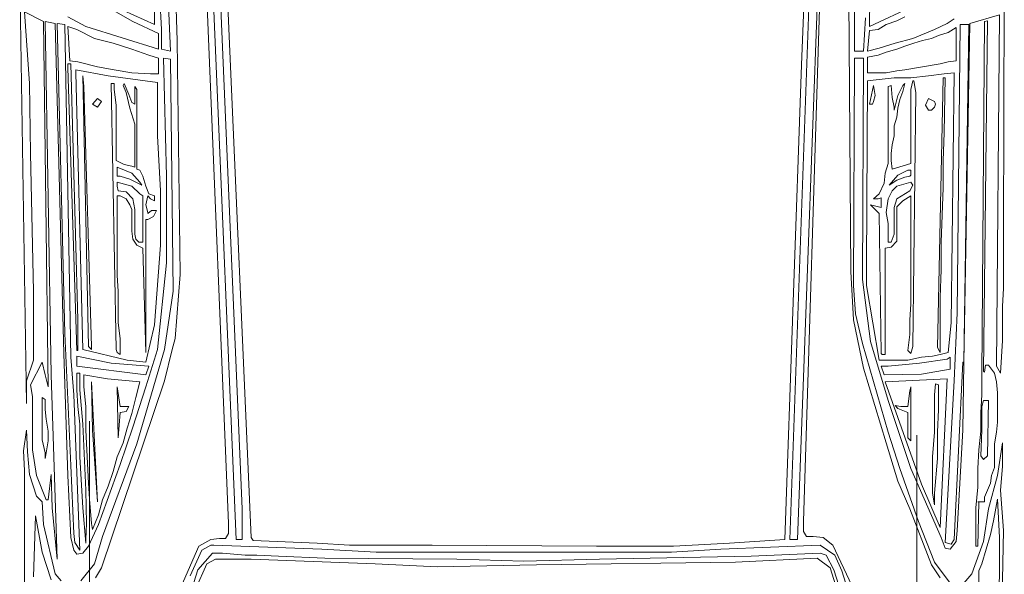
# Model space of a CAD drawing. Units: inches. Extents: x -36302355 to 648, y -221479757 to 75.
# Tile 6 of 37: x 185 to 225, y -507 to -484. Entities that reach past the tile are written whole.
import ezdxf

# ---------------------------------------------------------------- set-up
doc = ezdxf.new("R2010")
doc.units = ezdxf.units.IN
doc.header["$MEASUREMENT"] = 0
doc.layers.add('A-EQPM-VEHC', color=8, linetype='Continuous', lineweight=13)

msp = doc.modelspace()

# ---------------------------------------------------------------- linework, layer by layer
at = {"layer": 'A-EQPM-VEHC'}
for p, q in [((190.848, -484.778), (190.416, -476.638)), ((190.848, -476.717), (191.202, -485.643)), ((191.281, -479.233), (191.478, -485.211)), ((219.16, -480.61), (219.122, -484.66)), ((216.802, -480.963), (215.937, -505.148)), ((193.405, -481.554), (194.426, -505.069)), ((216.251, -505.148), (217.116, -481.672)), ((216.409, -486.194), (216.605, -481.358)), ((218.532, -485.643), (218.532, -481.318)), ((185.186, -482.655), (185.461, -499.721)), ((224.47, -492.957), (224.509, -482.772)), ((189.708, -484.464), (187.112, -482.969)), ((218.295, -483.165), (218.374, -494.452)), ((193.522, -504.518), (192.657, -483.323)), ((194.073, -503.929), (193.208, -483.599)), ((216.486, -504.439), (217.155, -483.285)), ((188.921, -483.834), (190.573, -484.581)), ((190.573, -484.581), (190.573, -483.953)), ((192.933, -484.03), (193.836, -505.148)), ((219.122, -484.66), (220.89, -483.834)), ((185.579, -486.941), (185.382, -484.071)), ((185.382, -484.071), (186.13, -484.464)), ((187.112, -484.267), (187.821, -484.66)), ((218.964, -484.306), (218.885, -485.643)), ((219.79, -484.581), (220.222, -484.425)), ((220.222, -484.425), (220.538, -484.267)), ((222.503, -484.346), (222.228, -484.543)), ((223.133, -484.543), (224.312, -484.188)), ((223.682, -498.423), (223.84, -484.425)), ((223.84, -484.425), (223.722, -484.464)), ((224.312, -484.188), (224.194, -498.226)), ((186.13, -484.464), (186.326, -499.052)), ((186.444, -498.58), (186.209, -484.464)), ((186.209, -484.464), (186.602, -484.543)), ((186.602, -484.543), (186.954, -497.715)), ((186.995, -484.581), (186.681, -484.543)), ((186.681, -484.543), (186.995, -496.929)), ((187.23, -497.873), (186.995, -484.581)), ((187.467, -484.778), (187.112, -484.66)), ((187.112, -484.66), (187.191, -486.036)), ((188.174, -485.132), (187.467, -484.778)), ((187.821, -484.66), (190.73, -485.564)), ((190.73, -484.936), (189.708, -484.464)), ((190.848, -485.564), (190.848, -484.778)), ((219.043, -485.643), (219.122, -484.818)), ((219.122, -484.818), (219.476, -484.778)), ((219.476, -484.778), (219.79, -484.581)), ((221.717, -484.778), (220.852, -485.132)), ((222.228, -484.543), (221.717, -484.778)), ((222.582, -484.699), (222.268, -484.895)), ((222.582, -486.036), (222.582, -484.699)), ((222.621, -496.103), (222.74, -484.581)), ((222.74, -484.581), (223.093, -484.581)), ((222.896, -498.07), (223.133, -484.543)), ((223.093, -484.581), (222.896, -498.07)), ((223.722, -484.464), (223.605, -498.58)), ((188.921, -485.329), (188.174, -485.132)), ((190.73, -485.564), (190.73, -484.936)), ((191.478, -485.211), (191.596, -494.569)), ((220.852, -485.132), (220.145, -485.329)), ((221.245, -485.211), (220.89, -485.329)), ((221.599, -485.132), (221.245, -485.211)), ((221.875, -485.015), (221.599, -485.132)), ((222.268, -484.895), (221.875, -485.015)), ((189.669, -485.564), (188.921, -485.329)), ((190.337, -485.801), (189.669, -485.564)), ((191.202, -485.643), (190.848, -485.564)), ((219.515, -485.525), (219.043, -485.643)), ((220.145, -485.329), (219.515, -485.525)), ((220.222, -485.564), (219.79, -485.683)), ((220.538, -485.446), (220.222, -485.564)), ((220.89, -485.329), (220.538, -485.446)), ((190.73, -485.918), (190.337, -485.801)), ((190.73, -486.548), (190.73, -485.918)), ((191.045, -490.637), (190.927, -485.918)), ((190.927, -485.918), (191.202, -485.959)), ((191.202, -485.959), (191.32, -495.238)), ((218.492, -495.002), (218.532, -485.918)), ((218.885, -485.643), (218.532, -485.643)), ((218.532, -485.918), (218.885, -485.918)), ((218.885, -485.918), (218.846, -494.766)), ((219.476, -485.801), (219.043, -485.88)), ((219.043, -485.88), (219.043, -486.508)), ((219.79, -485.683), (219.476, -485.801)), ((187.23, -486.155), (187.112, -486.155)), ((187.112, -486.155), (187.112, -486.311)), ((187.112, -486.311), (187.467, -497.598)), ((187.191, -486.036), (187.505, -486.076)), ((187.505, -496.378), (187.23, -486.155)), ((188.725, -486.626), (187.426, -486.39)), ((187.426, -486.39), (187.426, -486.508)), ((187.505, -486.076), (188.292, -486.273)), ((188.292, -486.273), (188.96, -486.39)), ((188.96, -486.39), (189.669, -486.508)), ((215.74, -505.148), (216.409, -486.194)), ((220.222, -486.429), (220.538, -486.39)), ((220.538, -486.39), (221.952, -486.155)), ((221.952, -486.155), (222.268, -486.076)), ((222.268, -486.076), (222.582, -486.036)), ((187.426, -486.508), (187.702, -497.557)), ((187.742, -487.059), (187.702, -486.626)), ((187.702, -486.626), (187.939, -497.44)), ((190.69, -486.901), (188.725, -486.626)), ((189.669, -486.508), (190.416, -486.548)), ((190.416, -486.548), (190.73, -486.548)), ((219.043, -486.508), (219.79, -486.508)), ((219.397, -486.783), (219.043, -486.824)), ((220.104, -486.705), (219.397, -486.783)), ((219.79, -486.508), (220.222, -486.429)), ((220.773, -486.705), (220.104, -486.705)), ((221.48, -486.626), (220.773, -486.705)), ((222.11, -486.548), (221.48, -486.626)), ((222.071, -486.705), (221.952, -492.407)), ((222.149, -486.705), (222.071, -486.705)), ((222.503, -486.508), (222.11, -486.548)), ((222.11, -488.907), (222.149, -486.705)), ((222.385, -496.496), (222.503, -486.508)), ((185.619, -489.733), (185.579, -486.941)), ((188.056, -497.44), (187.742, -487.059)), ((188.96, -486.941), (188.842, -486.941)), ((188.842, -486.941), (189.039, -497.557)), ((188.96, -487.177), (188.96, -486.941)), ((189.039, -487.806), (188.96, -487.177)), ((189.355, -486.941), (189.314, -487.02)), ((189.314, -487.02), (189.432, -487.294)), ((189.551, -487.373), (189.355, -486.941)), ((189.865, -487.177), (189.786, -487.059)), ((189.786, -487.059), (189.786, -487.766)), ((189.865, -490.361), (189.865, -487.177)), ((190.69, -489.024), (190.69, -486.901)), ((219.043, -486.824), (219.004, -494.216)), ((219.279, -487.02), (219.122, -487.766)), ((219.357, -487.413), (219.279, -487.02)), ((219.987, -487.02), (219.869, -487.059)), ((219.869, -487.059), (219.869, -490.126)), ((220.025, -487.492), (219.987, -487.02)), ((220.459, -487.02), (220.262, -487.413)), ((220.459, -487.255), (220.538, -486.941)), ((220.538, -486.941), (220.459, -487.02)), ((220.852, -486.824), (220.773, -487.177)), ((220.773, -487.177), (220.773, -490.126)), ((220.89, -486.824), (220.852, -486.824)), ((220.969, -487.294), (220.89, -486.824)), ((188.292, -487.531), (188.095, -487.766)), ((188.449, -487.649), (188.292, -487.531)), ((189.432, -487.294), (189.59, -487.924)), ((189.669, -487.689), (189.551, -487.373)), ((219.279, -487.649), (219.357, -487.413)), ((220.104, -487.885), (220.025, -487.492)), ((220.262, -487.413), (220.104, -488.003)), ((220.262, -487.924), (220.341, -487.57)), ((220.341, -487.57), (220.459, -487.255)), ((220.852, -497.44), (220.969, -487.294)), ((221.48, -487.531), (221.362, -487.806)), ((221.717, -487.649), (221.48, -487.531)), ((188.095, -487.766), (188.292, -487.885)), ((188.292, -487.885), (188.449, -487.649)), ((189.039, -490.009), (189.039, -487.806)), ((189.59, -487.924), (189.786, -488.554)), ((189.786, -487.766), (189.669, -487.689)), ((219.122, -487.766), (219.239, -487.766)), ((219.239, -487.766), (219.279, -487.649)), ((220.104, -488.003), (220.104, -487.885)), ((220.222, -488.278), (220.262, -487.924)), ((221.362, -487.806), (221.48, -488.003)), ((221.599, -488.003), (221.717, -487.885)), ((221.756, -487.766), (221.717, -487.649)), ((221.717, -487.885), (221.756, -487.766)), ((220.104, -488.631), (220.222, -488.278)), ((221.48, -488.003), (221.599, -488.003)), ((189.786, -488.554), (189.786, -490.284)), ((220.104, -489.024), (220.104, -488.631)), ((190.809, -491.226), (190.69, -489.024)), ((220.025, -489.379), (220.104, -489.024)), ((222.071, -490.009), (222.11, -488.907)), ((219.987, -489.733), (220.025, -489.379)), ((185.737, -495.238), (185.619, -489.733)), ((219.987, -490.009), (219.987, -489.733)), ((189.355, -490.165), (189.039, -490.009)), ((189.669, -490.519), (189.079, -490.284)), ((189.079, -490.284), (189.079, -490.637)), ((189.669, -490.244), (189.355, -490.165)), ((189.786, -490.284), (189.669, -490.244)), ((219.869, -490.126), (219.75, -490.519)), ((220.025, -490.361), (219.987, -490.009)), ((220.773, -490.126), (220.025, -490.361)), ((222.071, -491.109), (222.071, -490.009)), ((189.079, -490.637), (189.197, -490.637)), ((189.197, -490.637), (189.59, -490.756)), ((189.983, -490.874), (189.669, -490.519)), ((189.983, -490.402), (189.865, -490.361)), ((190.101, -490.637), (189.983, -490.402)), ((190.22, -491.03), (190.101, -490.637)), ((191.045, -494.097), (191.045, -490.637)), ((219.75, -490.519), (219.711, -490.912)), ((220.262, -490.598), (219.908, -490.991)), ((220.222, -490.795), (220.538, -490.677)), ((220.655, -490.402), (220.262, -490.598)), ((220.538, -490.677), (220.734, -490.637)), ((220.773, -490.402), (220.655, -490.402)), ((220.734, -490.637), (220.773, -490.598)), ((220.773, -490.598), (220.773, -490.402)), ((189.669, -491.03), (189.079, -490.874)), ((189.079, -490.874), (189.079, -491.03)), ((189.079, -491.03), (189.118, -491.226)), ((189.59, -490.756), (190.062, -490.991)), ((189.983, -491.346), (189.669, -491.03)), ((190.062, -490.991), (189.983, -490.874)), ((190.337, -491.346), (190.22, -491.03)), ((219.711, -490.912), (219.515, -491.346)), ((219.908, -490.991), (220.222, -490.795)), ((220.222, -491.03), (220.025, -491.226)), ((220.773, -490.874), (220.222, -491.03)), ((220.734, -491.226), (220.852, -490.991)), ((220.852, -490.991), (220.773, -490.874)), ((221.992, -493.272), (222.071, -491.109)), ((189.079, -494.609), (189.079, -491.425)), ((189.079, -491.425), (189.197, -491.425)), ((189.118, -491.226), (189.432, -491.267)), ((189.197, -491.425), (189.432, -491.542)), ((189.432, -491.267), (189.708, -491.542)), ((190.101, -491.425), (189.983, -491.346)), ((190.101, -493.272), (190.101, -491.425)), ((190.22, -491.777), (190.297, -491.425)), ((190.297, -491.425), (190.416, -491.542)), ((190.573, -491.425), (190.337, -491.346)), ((190.573, -491.621), (190.573, -491.425)), ((190.809, -493.39), (190.809, -491.226)), ((219.515, -491.346), (219.279, -491.542)), ((219.476, -491.542), (219.594, -491.502)), ((219.594, -491.502), (219.594, -491.895)), ((220.025, -491.226), (219.869, -491.542)), ((220.222, -491.542), (220.734, -491.226)), ((220.459, -491.621), (220.773, -491.425)), ((220.773, -491.425), (220.773, -495.75)), ((189.432, -491.542), (189.59, -491.777)), ((189.59, -491.777), (189.669, -491.974)), ((189.708, -491.542), (189.786, -491.974)), ((190.297, -492.092), (190.22, -491.777)), ((190.416, -491.542), (190.573, -491.621)), ((219.594, -491.895), (219.16, -491.777)), ((219.16, -491.777), (219.515, -492.132)), ((219.279, -491.542), (219.476, -491.542)), ((219.869, -491.542), (219.79, -492.092)), ((220.104, -491.895), (220.222, -491.542)), ((220.104, -492.957), (220.104, -491.895)), ((220.222, -491.856), (220.459, -491.621)), ((220.222, -493.232), (220.222, -491.856)), ((189.669, -491.974), (189.669, -492.839)), ((189.786, -491.974), (189.786, -492.957)), ((190.455, -492.014), (190.297, -492.132)), ((190.297, -492.132), (190.297, -492.092)), ((190.297, -492.367), (190.534, -492.249)), ((190.652, -492.014), (190.455, -492.014)), ((190.534, -492.249), (190.652, -492.014)), ((219.515, -492.132), (219.594, -497.715)), ((219.79, -492.092), (219.869, -492.525)), ((190.22, -497.677), (190.22, -492.367)), ((190.22, -492.367), (190.297, -492.367)), ((219.869, -492.525), (219.869, -493.272)), ((221.952, -492.407), (221.834, -497.48)), ((189.669, -492.839), (189.708, -493.155)), ((189.786, -492.957), (189.825, -493.155)), ((219.987, -493.272), (220.104, -492.957)), ((224.47, -495.12), (224.47, -492.957)), ((189.708, -493.155), (189.865, -493.39)), ((189.825, -493.155), (189.944, -493.272)), ((189.865, -493.39), (190.101, -493.508)), ((189.944, -493.272), (190.101, -493.272)), ((190.573, -496.575), (190.809, -493.39)), ((219.75, -493.508), (219.987, -493.469)), ((219.869, -493.272), (219.987, -493.272)), ((219.987, -493.469), (220.222, -493.232)), ((221.992, -494.373), (221.992, -493.272)), ((190.101, -493.508), (190.22, -497.677)), ((219.75, -497.756), (219.75, -493.508)), ((190.69, -497.557), (191.045, -494.097)), ((219.004, -494.216), (219.004, -495.002)), ((189.118, -495.238), (189.079, -494.609)), ((191.596, -494.569), (191.399, -497.126)), ((218.374, -494.452), (218.492, -496.378)), ((221.952, -495.474), (221.992, -494.373)), ((218.571, -496.143), (218.492, -495.002)), ((218.846, -494.766), (219.16, -497.243)), ((219.004, -495.002), (219.515, -497.991)), ((185.737, -497.991), (185.737, -495.238)), ((189.118, -496.496), (189.118, -495.238)), ((191.32, -495.238), (190.966, -497.557)), ((224.43, -495.827), (224.47, -495.12)), ((220.773, -495.75), (220.734, -496.378)), ((221.952, -497.677), (221.952, -495.474)), ((224.43, -497.205), (224.43, -495.827)), ((218.846, -497.322), (218.571, -496.143)), ((222.503, -498.817), (222.621, -496.103)), ((187.505, -497.598), (187.505, -496.378)), ((189.197, -497.126), (189.118, -496.496)), ((190.22, -498.07), (190.573, -496.575)), ((218.492, -496.378), (218.885, -498.305)), ((220.734, -496.378), (220.734, -496.968)), ((222.268, -497.677), (222.385, -496.496)), ((186.995, -496.929), (187.23, -502.199)), ((220.734, -496.968), (220.655, -497.598)), ((189.197, -497.756), (189.197, -497.126)), ((191.399, -497.126), (191.281, -497.557)), ((219.869, -500.861), (218.846, -497.322)), ((219.16, -497.243), (219.869, -499.603)), ((224.351, -498.501), (224.43, -497.205)), ((186.954, -497.715), (187.112, -502.592)), ((187.467, -497.598), (187.505, -497.598)), ((187.702, -497.557), (189.472, -497.991)), ((187.939, -497.44), (188.056, -497.557)), ((188.056, -497.557), (188.056, -497.44)), ((189.039, -497.557), (189.079, -497.677)), ((189.079, -497.677), (189.197, -497.756)), ((190.966, -497.557), (189.865, -501.333)), ((190.22, -499.052), (190.69, -497.557)), ((191.281, -497.557), (190.966, -498.817)), ((219.594, -497.715), (219.632, -497.756)), ((219.632, -497.756), (219.75, -497.756)), ((220.655, -497.598), (220.773, -497.715)), ((220.773, -497.715), (220.852, -497.44)), ((221.638, -497.833), (221.952, -497.756)), ((221.834, -497.48), (221.952, -497.677)), ((221.952, -497.756), (222.268, -497.677)), ((185.461, -498.817), (185.737, -497.991)), ((186.089, -498.07), (185.619, -498.973)), ((186.209, -498.58), (186.089, -498.07)), ((187.349, -499.367), (187.23, -497.873)), ((188.842, -498.108), (187.467, -497.833)), ((187.467, -497.833), (187.467, -498.226)), ((190.337, -498.226), (188.842, -498.108)), ((189.472, -497.991), (190.22, -498.07)), ((219.515, -497.991), (220.655, -497.991)), ((221.127, -498.108), (219.869, -498.226)), ((220.655, -497.991), (221.206, -497.873)), ((222.228, -497.952), (221.127, -498.108)), ((221.206, -497.873), (221.638, -497.833)), ((222.345, -497.873), (222.228, -497.952)), ((222.345, -498.345), (222.345, -497.873)), ((222.857, -498.07), (222.503, -505.148)), ((222.896, -498.07), (222.857, -498.07)), ((222.857, -500.783), (222.896, -498.108)), ((222.896, -498.108), (222.896, -498.07)), ((223.761, -498.187), (223.722, -498.463)), ((223.879, -498.187), (223.761, -498.187)), ((224.116, -498.501), (223.879, -498.187)), ((186.326, -499.052), (186.209, -498.58)), ((186.681, -505.934), (186.444, -498.58)), ((187.467, -498.226), (190.22, -498.58)), ((187.584, -498.501), (187.467, -498.501)), ((187.467, -498.501), (187.467, -499.17)), ((187.584, -499.17), (187.584, -498.501)), ((188.686, -498.738), (187.742, -498.58)), ((187.742, -498.58), (187.742, -499.052)), ((190.22, -498.58), (190.337, -498.226)), ((218.885, -498.305), (219.79, -501.293)), ((219.869, -498.226), (219.594, -498.226)), ((219.594, -498.226), (219.711, -498.58)), ((219.711, -498.58), (221.206, -498.542)), ((221.206, -498.542), (222.345, -498.345)), ((223.605, -498.58), (223.605, -499.367)), ((223.722, -498.463), (223.682, -498.423)), ((224.194, -498.856), (224.116, -498.501)), ((224.194, -498.226), (224.351, -498.501)), ((185.461, -499.721), (185.461, -498.817)), ((185.619, -498.973), (185.696, -499.445)), ((188.292, -503.653), (188.056, -498.856)), ((188.056, -498.856), (188.095, -500.783)), ((190.966, -498.817), (188.449, -506.287)), ((189.983, -498.856), (188.686, -498.738)), ((189.825, -499.486), (189.983, -498.856)), ((222.228, -498.738), (219.75, -498.856)), ((219.75, -498.856), (221.206, -502.946)), ((221.756, -498.935), (221.717, -499.367)), ((221.875, -498.973), (221.756, -498.935)), ((221.875, -499.956), (221.875, -498.973)), ((221.952, -504.676), (222.228, -498.738)), ((222.149, -505.266), (222.503, -498.817)), ((224.233, -499.289), (224.194, -498.856)), ((187.584, -505.58), (187.349, -499.367)), ((187.467, -499.17), (187.505, -499.839)), ((187.702, -500.547), (187.584, -499.17)), ((187.742, -499.052), (187.821, -499.839)), ((189.197, -499.839), (189.079, -499.052)), ((189.079, -499.052), (189.118, -501.097)), ((189.708, -500.665), (190.22, -499.052)), ((220.734, -499.21), (220.655, -499.839)), ((220.773, -499.052), (220.734, -499.21)), ((220.773, -501.216), (220.773, -499.052)), ((221.717, -499.367), (221.717, -500.861)), ((223.605, -499.367), (223.565, -500.075)), ((224.233, -500.468), (224.233, -499.289)), ((185.696, -499.445), (185.696, -501.569)), ((186.209, -499.563), (186.089, -499.486)), ((186.089, -499.486), (186.089, -501.176)), ((186.209, -499.956), (186.209, -499.563)), ((189.669, -500.114), (189.825, -499.486)), ((219.869, -499.603), (220.773, -502.316)), ((223.682, -499.603), (223.605, -499.839)), ((223.879, -499.603), (223.682, -499.603)), ((223.84, -501.805), (223.879, -499.603)), ((186.247, -500.351), (186.209, -499.956)), ((187.505, -499.839), (187.584, -500.547)), ((187.821, -499.839), (187.821, -500.783)), ((189.118, -501.097), (189.197, -500.075)), ((189.551, -499.839), (189.197, -499.839)), ((189.197, -500.075), (189.432, -500.035)), ((189.432, -500.035), (189.551, -499.839)), ((189.472, -500.704), (189.669, -500.114)), ((220.38, -499.839), (220.145, -499.8)), ((220.145, -499.8), (220.262, -499.917)), ((220.262, -499.917), (220.655, -500.075)), ((220.655, -499.839), (220.38, -499.839)), ((220.655, -500.075), (220.655, -501.097)), ((221.834, -500.861), (221.875, -499.956)), ((223.565, -500.075), (223.565, -500.821)), ((223.605, -499.839), (223.605, -500.783)), ((186.326, -500.821), (186.247, -500.351)), ((187.584, -500.547), (187.584, -501.844)), ((187.821, -503.181), (187.702, -500.547)), ((187.977, -500.428), (187.977, -514.82)), ((224.194, -500.861), (224.233, -500.468)), ((185.461, -500.783), (185.343, -501.609)), ((185.5, -501.648), (185.461, -500.783)), ((186.326, -501.216), (186.326, -500.821)), ((187.821, -500.783), (187.939, -502.906)), ((188.095, -500.783), (188.292, -503.653)), ((189.197, -502.158), (189.708, -500.665)), ((189.314, -501.293), (189.472, -500.704)), ((220.341, -502.316), (219.869, -500.861)), ((221.717, -500.861), (221.638, -501.844)), ((221.834, -501.923), (221.834, -500.861)), ((222.621, -504.794), (222.857, -500.783)), ((223.565, -500.821), (223.486, -501.569)), ((223.605, -500.783), (223.565, -501.805)), ((224.116, -501.333), (224.194, -500.861)), ((186.089, -501.176), (186.209, -501.688)), ((186.247, -501.688), (186.326, -501.216)), ((189.865, -501.333), (188.488, -505.029)), ((189.079, -501.844), (189.314, -501.293)), ((219.79, -501.293), (220.262, -502.827)), ((220.655, -501.097), (220.773, -501.216)), ((221.01, -500.979), (221.01, -515.45)), ((224.116, -502.277), (224.116, -501.333)), ((224.43, -501.293), (224.233, -502.592)), ((224.43, -502.237), (224.43, -501.293)), ((185.343, -501.609), (185.382, -502.395)), ((185.579, -502.553), (185.5, -501.648)), ((185.696, -501.569), (185.854, -502.592)), ((186.209, -501.923), (186.247, -501.688)), ((186.209, -501.688), (186.209, -501.923)), ((223.486, -501.569), (223.447, -502.316)), ((187.584, -501.844), (187.702, -503.888)), ((188.921, -502.434), (189.079, -501.844)), ((221.638, -501.844), (221.638, -503.299)), ((221.717, -503.299), (221.834, -501.923)), ((223.565, -501.805), (223.682, -501.962)), ((223.682, -501.962), (223.84, -501.805)), ((185.382, -502.395), (185.382, -509.277)), ((187.23, -502.199), (187.349, -504.911)), ((188.332, -504.557), (189.197, -502.158)), ((188.725, -503.023), (188.921, -502.434)), ((221.087, -504.439), (220.341, -502.316)), ((220.773, -502.316), (221.992, -505.069)), ((223.447, -502.316), (223.447, -503.064)), ((223.998, -502.592), (224.116, -502.277)), ((224.351, -503.181), (224.43, -502.237)), ((185.854, -503.418), (185.579, -502.553)), ((185.854, -502.592), (186.247, -503.574)), ((186.326, -503.574), (186.444, -502.553)), ((186.444, -502.553), (186.484, -503.888)), ((187.112, -502.592), (187.23, -505.069)), ((187.939, -502.906), (187.977, -503.536)), ((220.262, -502.827), (220.734, -503.929)), ((223.722, -503.457), (223.958, -502.906)), ((224.233, -502.592), (223.879, -503.929)), ((223.958, -502.906), (223.998, -502.592)), ((187.86, -504.518), (187.821, -503.181)), ((188.488, -503.574), (188.725, -503.023)), ((221.206, -502.946), (221.952, -504.676)), ((221.638, -503.299), (221.717, -503.771)), ((221.717, -503.771), (221.717, -503.299)), ((223.447, -503.064), (223.368, -503.888)), ((224.47, -504.794), (224.351, -503.181)), ((186.089, -503.653), (185.854, -503.418)), ((186.13, -504.557), (186.089, -503.653)), ((186.247, -503.574), (186.326, -503.574)), ((187.977, -503.536), (188.056, -504.518)), ((188.332, -504.164), (188.488, -503.574)), ((223.447, -505.422), (223.486, -503.653)), ((223.447, -503.653), (223.722, -503.653)), ((223.722, -503.653), (223.722, -503.457)), ((224.077, -504.401), (224.233, -503.536)), ((224.233, -503.536), (224.312, -505.069)), ((186.484, -503.888), (186.681, -505.934)), ((187.702, -503.888), (187.821, -505.304)), ((194.073, -505.148), (194.073, -503.929)), ((220.734, -503.929), (221.599, -506.17)), ((223.368, -503.888), (223.368, -505.422)), ((223.879, -503.929), (223.682, -505.226)), ((185.815, -504.204), (185.737, -506.642)), ((185.972, -505.069), (185.815, -504.204)), ((188.095, -504.754), (188.332, -504.164)), ((216.486, -504.832), (216.486, -504.439)), ((221.717, -506.052), (221.087, -504.439)), ((223.958, -504.952), (224.077, -504.401)), ((186.602, -506.524), (186.13, -504.557)), ((187.821, -505.148), (187.86, -504.518)), ((187.939, -505.422), (188.332, -504.557)), ((188.056, -504.518), (188.095, -504.754)), ((193.522, -504.911), (193.522, -504.518)), ((216.605, -505.029), (216.486, -504.832)), ((222.582, -505.226), (222.621, -504.794)), ((224.312, -512.579), (224.47, -504.794)), ((186.089, -505.659), (185.972, -505.069)), ((187.23, -505.069), (187.349, -505.58)), ((187.349, -504.911), (187.388, -505.266)), ((187.388, -505.266), (187.584, -505.58)), ((187.821, -505.304), (187.821, -505.148)), ((188.488, -505.029), (188.174, -506.131)), ((192.343, -505.422), (192.815, -505.148)), ((192.815, -505.148), (193.168, -505.108)), ((193.168, -505.108), (193.405, -505.108)), ((193.405, -505.108), (193.522, -504.911)), ((193.836, -505.148), (194.073, -505.148)), ((194.426, -505.069), (194.505, -505.187)), ((194.505, -505.187), (197.061, -505.304)), ((213.538, -505.304), (215.74, -505.148)), ((215.937, -505.148), (216.251, -505.148)), ((216.881, -505.029), (216.605, -505.029)), ((217.274, -505.069), (216.881, -505.029)), ((217.667, -505.383), (217.274, -505.069)), ((221.992, -505.069), (222.149, -505.501)), ((222.385, -505.345), (222.149, -505.266)), ((222.345, -505.541), (222.582, -505.226)), ((222.503, -505.148), (222.385, -505.345)), ((223.682, -505.226), (223.212, -506.524)), ((223.605, -506.131), (223.958, -504.952)), ((224.312, -505.069), (224.312, -506.524)), ((186.444, -506.759), (186.089, -505.659)), ((187.349, -505.58), (187.467, -505.738)), ((187.702, -505.698), (187.939, -505.422)), ((191.634, -507.035), (192.343, -505.422)), ((192.461, -505.58), (191.989, -506.603)), ((192.815, -505.383), (192.461, -505.58)), ((192.933, -505.383), (192.815, -505.383)), ((197.258, -505.541), (192.933, -505.383)), ((197.061, -505.304), (198.358, -505.383)), ((199.42, -505.659), (197.258, -505.541)), ((198.358, -505.383), (201.662, -505.383)), ((211.217, -505.659), (199.42, -505.659)), ((201.662, -505.383), (208.228, -505.422)), ((208.228, -505.422), (211.296, -505.422)), ((213.184, -505.541), (211.217, -505.659)), ((211.296, -505.422), (213.538, -505.304)), ((217.155, -505.383), (213.184, -505.541)), ((217.746, -505.776), (217.155, -505.383)), ((218.413, -506.996), (217.667, -505.383)), ((222.149, -505.501), (222.345, -505.541)), ((223.368, -505.422), (223.447, -505.422)), ((187.467, -505.738), (187.702, -505.698)), ((192.892, -505.698), (192.303, -506.366)), ((193.012, -505.934), (192.657, -506.131)), ((193.287, -505.698), (192.892, -505.698)), ((194.426, -505.934), (193.012, -505.934)), ((194.191, -505.776), (193.287, -505.698)), ((194.663, -505.776), (194.191, -505.776)), ((199.381, -506.131), (194.426, -505.934)), ((195.528, -505.817), (194.663, -505.776)), ((197.376, -505.894), (195.528, -505.817)), ((202.645, -505.934), (197.376, -505.894)), ((205.319, -506.013), (202.645, -505.934)), ((208.348, -505.934), (205.319, -506.013)), ((213.773, -506.052), (205.83, -506.17)), ((214.403, -505.817), (208.348, -505.934)), ((217.037, -505.894), (213.773, -506.052)), ((217.155, -505.698), (214.403, -505.817)), ((217.548, -506.287), (217.037, -505.894)), ((217.391, -505.776), (217.155, -505.698)), ((217.706, -506.366), (217.391, -505.776)), ((218.02, -506.406), (217.746, -505.776)), ((222.385, -506.956), (221.717, -506.052)), ((188.174, -506.131), (187.623, -506.799)), ((188.449, -506.287), (188.214, -506.682)), ((192.303, -506.366), (191.713, -508.175)), ((192.657, -506.131), (192.224, -507.114)), ((201.859, -506.248), (199.381, -506.131)), ((205.83, -506.17), (201.859, -506.248)), ((217.902, -507.389), (217.548, -506.287)), ((217.902, -506.996), (217.706, -506.366)), ((218.611, -508.293), (218.02, -506.406)), ((221.599, -506.17), (221.952, -506.682)), ((223.486, -506.406), (223.605, -506.131)), ((223.486, -506.996), (223.486, -506.406)), ((186.837, -506.799), (186.602, -506.524)), ((223.212, -506.524), (222.817, -506.996)), ((224.312, -506.524), (224.233, -509.474))]:
    msp.add_line(p, q, dxfattribs=at)

doc.saveas('drawing.dxf')
